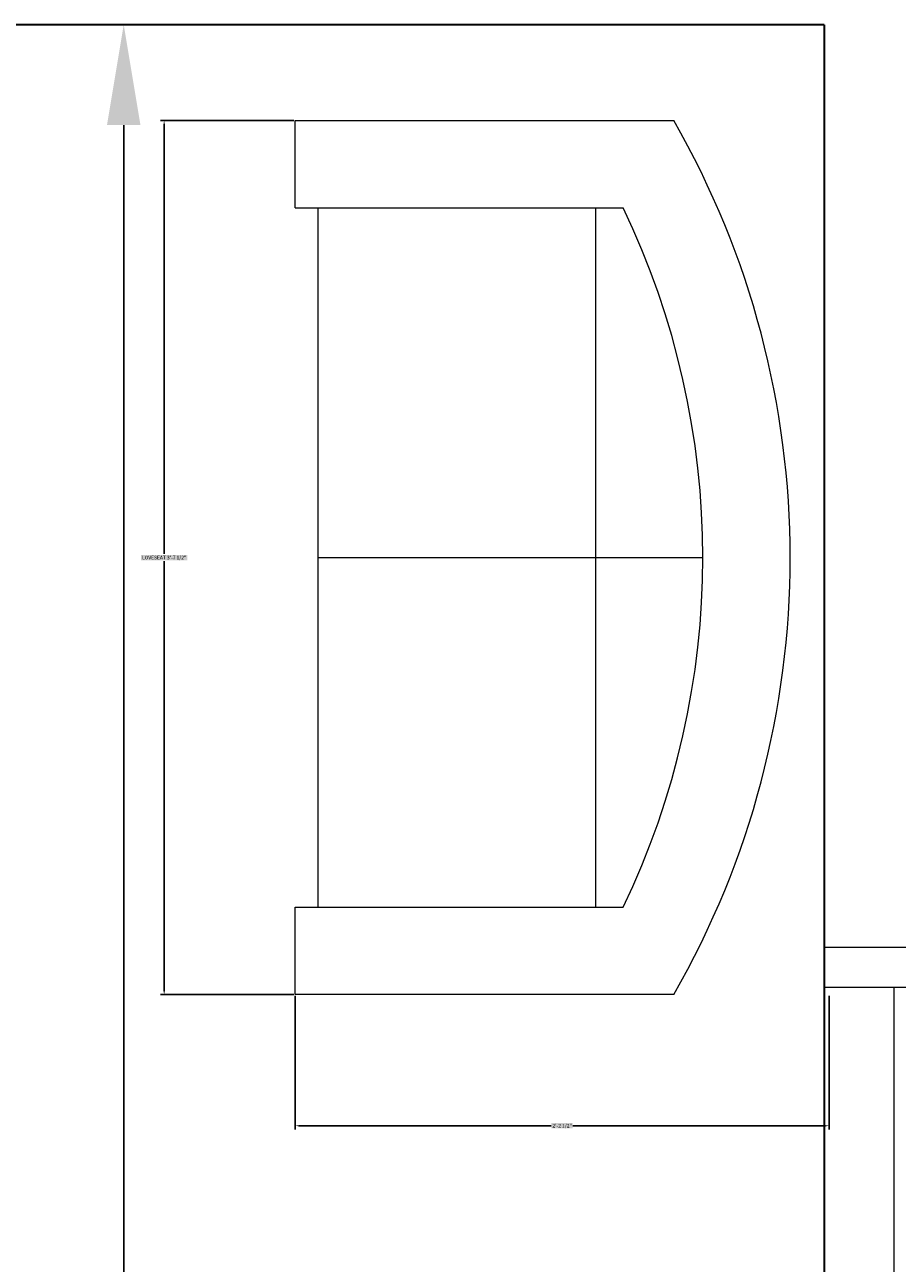
# Model space of a CAD drawing. Units: inches. Extents: x -128 to 854, y -395 to 398.
# Tile 31 of 61: x 265 to 309, y 2 to 64. Entities that reach past the tile are written whole.
import ezdxf

# ---------------------------------------------------------------- set-up
doc = ezdxf.new("R2010")
doc.units = ezdxf.units.IN
doc.header["$MEASUREMENT"] = 0
for name, color, linetype, lineweight in [('A-ANNO-DIMS', 2, 'Continuous', 18), ('A-FURN', 8, 'Continuous', 18), ('A-GLAZ', 220, 'Continuous', 18), ('A-WALL', 4, 'Continuous', 35)]:
    doc.layers.add(name, color=color, linetype=linetype, lineweight=lineweight)
doc.styles.get("Standard").update_dxf_attribs({"font": 'arial.ttf'})
doc.dimstyles.get("Standard").update_dxf_attribs({"dimtxt": 0.18, "dimasz": 0.18, "dimexe": 0.18, "dimexo": 0.0625, "dimgap": 0.09, "dimtad": 0, "dimtih": 1, "dimtoh": 1, "dimdec": 1, "dimzin": 0, "dimdsep": 46, "dimlunit": 4, "dimtxsty": 'Standard', "dimcen": 0.09, "dimclrd": 1, "dimclre": 2, "dimclrt": 6, "dimadec": 0, "dimazin": 0, "dimtfac": 1, "dimtdec": 1, "dimtofl": 0, "dimtmove": 0, "dimatfit": 3, "dimfxl": 1, "dimtfill": 2, "dimtfillclr": 3, "dimtolj": 1, "dimtzin": 0, "dimarcsym": 0})

# ---------------------------------------------------------------- blocks, each defined once
blk = doc.blocks.new('Sofa - Roundback Loveseat 5 ft.')
for p, q in [((0, -32.44198), (0, -5.99998)), ((-24, -33.99998), (-24, -11.46958)), ((24.00004, -33.99998), (24.00004, -11.46958)), ((-23.9998, -13.38178), (23.99986, -13.38178)), ((-24, -32.44198), (24.00004, -32.44198))]:
    blk.add_line(p, q)
for points in [[(-24, -33.99998), (-30, -33.99998), (-30, -7.99998)], [(30.00004, -7.99998), (30.00004, -33.99998), (24.00004, -33.99998)]]:
    blk.add_lwpolyline(points)
for centre, radius, start, end in [((0, -60.24998), 60.24998, 60.13715, 119.8628), ((0, -61.38438), 55.38444, 64.32083, 115.6792)]:
    blk.add_arc(centre, radius, start, end)
blk = doc.blocks.new('*D42')
at = {"layer": 'A-ANNO-DIMS', "color": 0, "lineweight": -2, "transparency": 16777216}
for p, q in [((304.81, 63.741), (269.747, 63.741)), ((269.927, 58.741), (269.927, -6.161)), ((269.927, -75.259), (269.927, -10.358)), ((304.81, -80.259), (269.747, -80.259))]:
    blk.add_line(p, q, dxfattribs=at)
at = {"layer": 'A-ANNO-DIMS', "color": 0, "transparency": 16777216}
for points in [[(269.093, 58.741), (270.76, 58.741), (269.927, 63.741)], [(269.093, -75.259), (270.76, -75.259), (269.927, -80.259)]]:
    blk.add_solid(points, dxfattribs=at)
at = {"layer": 'Defpoints', "color": 0, "transparency": 16777216}
for p in [(269.927, 63.741), (304.873, 63.741), (304.873, -80.259)]:
    blk.add_point(p, dxfattribs=at)
at = {"layer": 'A-ANNO-DIMS', "color": 0, "transparency": 16777216, "insert": (269.927, -8.259), "char_height": 4, "attachment_point": 5, "bg_fill": 1, "box_fill_scale": 1.25, "bg_fill_color": 3, "bg_fill_transparency": 0}
blk.add_mtext("\\A1;12'", dxfattribs=at)
blk = doc.blocks.new('WIN-48IN')
for p, q in [((9, 52), (0, 52)), ((9, 50), (0, 50)), ((3.5, 50), (3.5, 2)), ((5.5, 50), (5.5, 2)), ((9, 26), (0, 26)), ((9, 2), (0, 2)), ((9, 0), (0, 0))]:
    blk.add_line(p, q)
blk = doc.blocks.new('*D93')
at = {"layer": 'A-ANNO-DIMS', "color": 2, "lineweight": -2, "transparency": 16777216}
for p, q in [((278.42, 58.966), (271.764, 58.966)), ((278.42, 15.375), (271.764, 15.375))]:
    blk.add_line(p, q, dxfattribs=at)
at = {"layer": 'A-ANNO-DIMS', "color": 1, "lineweight": -2, "transparency": 16777216}
for p, q in [((271.944, 58.786), (271.944, 37.354)), ((271.944, 15.555), (271.944, 36.987))]:
    blk.add_line(p, q, dxfattribs=at)
at = {"layer": 'A-ANNO-DIMS', "color": 1, "transparency": 16777216}
for points in [[(271.914, 58.786), (271.974, 58.786), (271.944, 58.966)], [(271.914, 15.555), (271.974, 15.555), (271.944, 15.375)]]:
    blk.add_solid(points, dxfattribs=at)
at = {"layer": 'Defpoints', "color": 0, "transparency": 16777216}
for p in [(278.482, 58.966), (271.944, 15.375), (278.482, 15.375)]:
    blk.add_point(p, dxfattribs=at)
at = {"layer": 'A-ANNO-DIMS', "color": 6, "transparency": 16777216, "insert": (271.944, 37.17), "char_height": 0.18, "attachment_point": 5, "bg_fill": 1, "box_fill_scale": 1.25, "bg_fill_color": 3, "bg_fill_transparency": 0}
blk.add_mtext('\\A1;LOVESEAT 3\'-7 1/2"', dxfattribs=at)
blk = doc.blocks.new('*D94')
at = {"layer": 'A-ANNO-DIMS', "color": 2, "lineweight": -2, "transparency": 16777216}
for p, q in [((278.482, 15.313), (278.482, 8.657)), ((305.121, 15.313), (305.121, 8.657))]:
    blk.add_line(p, q, dxfattribs=at)
at = {"layer": 'A-ANNO-DIMS', "color": 1, "lineweight": -2, "transparency": 16777216}
for p, q in [((278.662, 8.837), (291.261, 8.837)), ((304.941, 8.837), (292.342, 8.837))]:
    blk.add_line(p, q, dxfattribs=at)
at = {"layer": 'A-ANNO-DIMS', "color": 1, "transparency": 16777216}
for points in [[(278.662, 8.867), (278.662, 8.807), (278.482, 8.837)], [(304.941, 8.867), (304.941, 8.807), (305.121, 8.837)]]:
    blk.add_solid(points, dxfattribs=at)
at = {"layer": 'Defpoints', "color": 0, "transparency": 16777216}
for p in [(278.482, 15.375), (305.121, 15.375), (305.121, 8.837)]:
    blk.add_point(p, dxfattribs=at)
at = {"layer": 'A-ANNO-DIMS', "color": 6, "transparency": 16777216, "insert": (291.801, 8.837), "char_height": 0.18, "attachment_point": 5, "bg_fill": 1, "box_fill_scale": 1.25, "bg_fill_color": 3, "bg_fill_transparency": 0}
blk.add_mtext('\\A1;2\'-2 1/2"', dxfattribs=at)

msp = doc.modelspace()

# ---------------------------------------------------------------- linework, layer by layer
at = {"layer": 'A-WALL'}
for q in [(196.76, 63.741), (304.873, -80.259)]:
    msp.add_line((304.873, 63.741), q, dxfattribs=at)

# ---------------------------------------------------------------- block references
at = {"layer": 'A-FURN', "xscale": 0.7265012871695607, "yscale": 0.7265012871695607, "zscale": 0.7265012871695607, "rotation": 270}
msp.add_blockref('Sofa - Roundback Loveseat 5 ft.', (303.183, 37.17), dxfattribs=at)
at = {"layer": 'A-GLAZ', "rotation": 180}
msp.add_blockref('WIN-48IN', (313.873, 17.741), dxfattribs=at)

# ---------------------------------------------------------------- dimensions: what is measured, and where the dimension line sits
at = {"layer": 'A-ANNO-DIMS'}
dim = msp.add_linear_dim(base=(269.927, 63.741), p1=(304.873, -80.259), p2=(304.873, 63.741), angle=90, dimstyle='Standard', override={"dimtxt": 4, "dimasz": 5, "dimclrd": 0, "dimclre": 0, "dimclrt": 0}, dxfattribs=at)
dim.commit()
dim.dimension.update_dxf_attribs({"geometry": '*D42', "text_midpoint": (269.927, -8.259)})
dim = msp.add_linear_dim(base=(271.944, 15.375), p1=(278.482, 58.966), p2=(278.482, 15.375), angle=270, text='LOVESEAT <>', dimstyle='Standard', override={"dimdec": 1, "dimlfac": 1, "dimrnd": 0, "dimzin": 1, "dimdsep": 46, "dimlunit": 4, "dimfrac": 2}, dxfattribs=at)
dim.commit()
dim.dimension.update_dxf_attribs({"geometry": '*D93', "text_midpoint": (271.944, 37.17)})
dim = msp.add_linear_dim(base=(305.121, 8.837), p1=(278.482, 15.375), p2=(305.121, 15.375), dimstyle='Standard', override={"dimdec": 1, "dimlfac": 1, "dimrnd": 0, "dimzin": 1, "dimdsep": 46, "dimlunit": 4, "dimfrac": 2}, dxfattribs=at)
dim.commit()
dim.dimension.update_dxf_attribs({"geometry": '*D94', "text_midpoint": (291.801, 8.837)})

doc.saveas('drawing.dxf')
